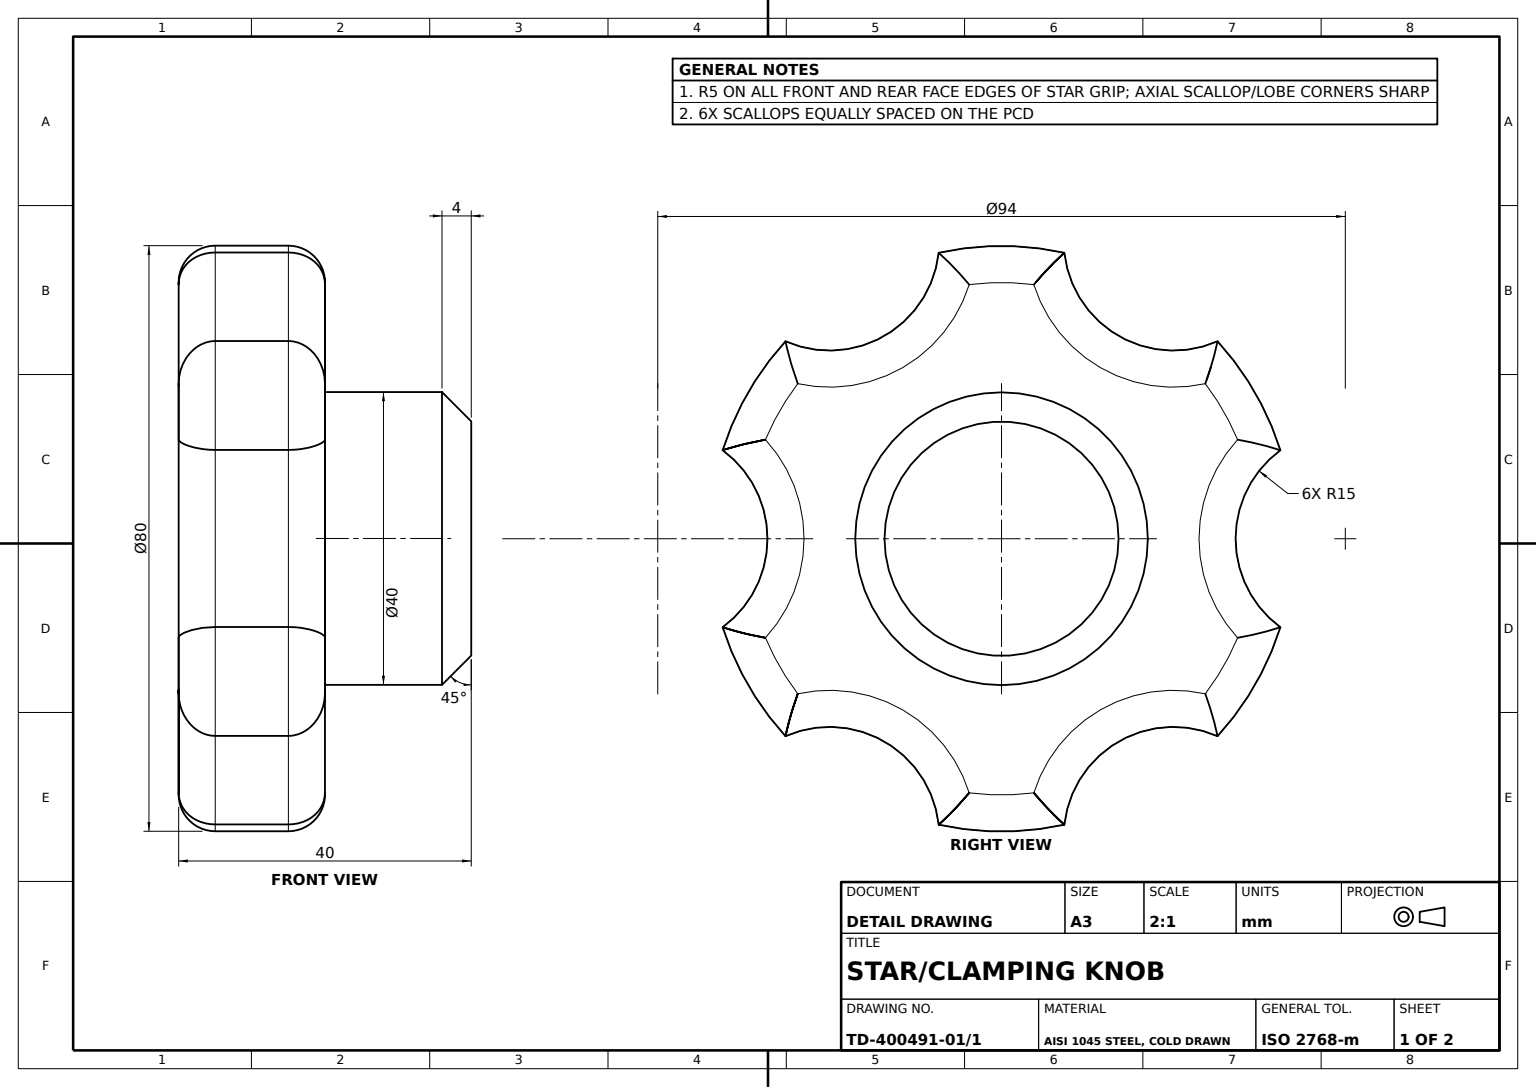
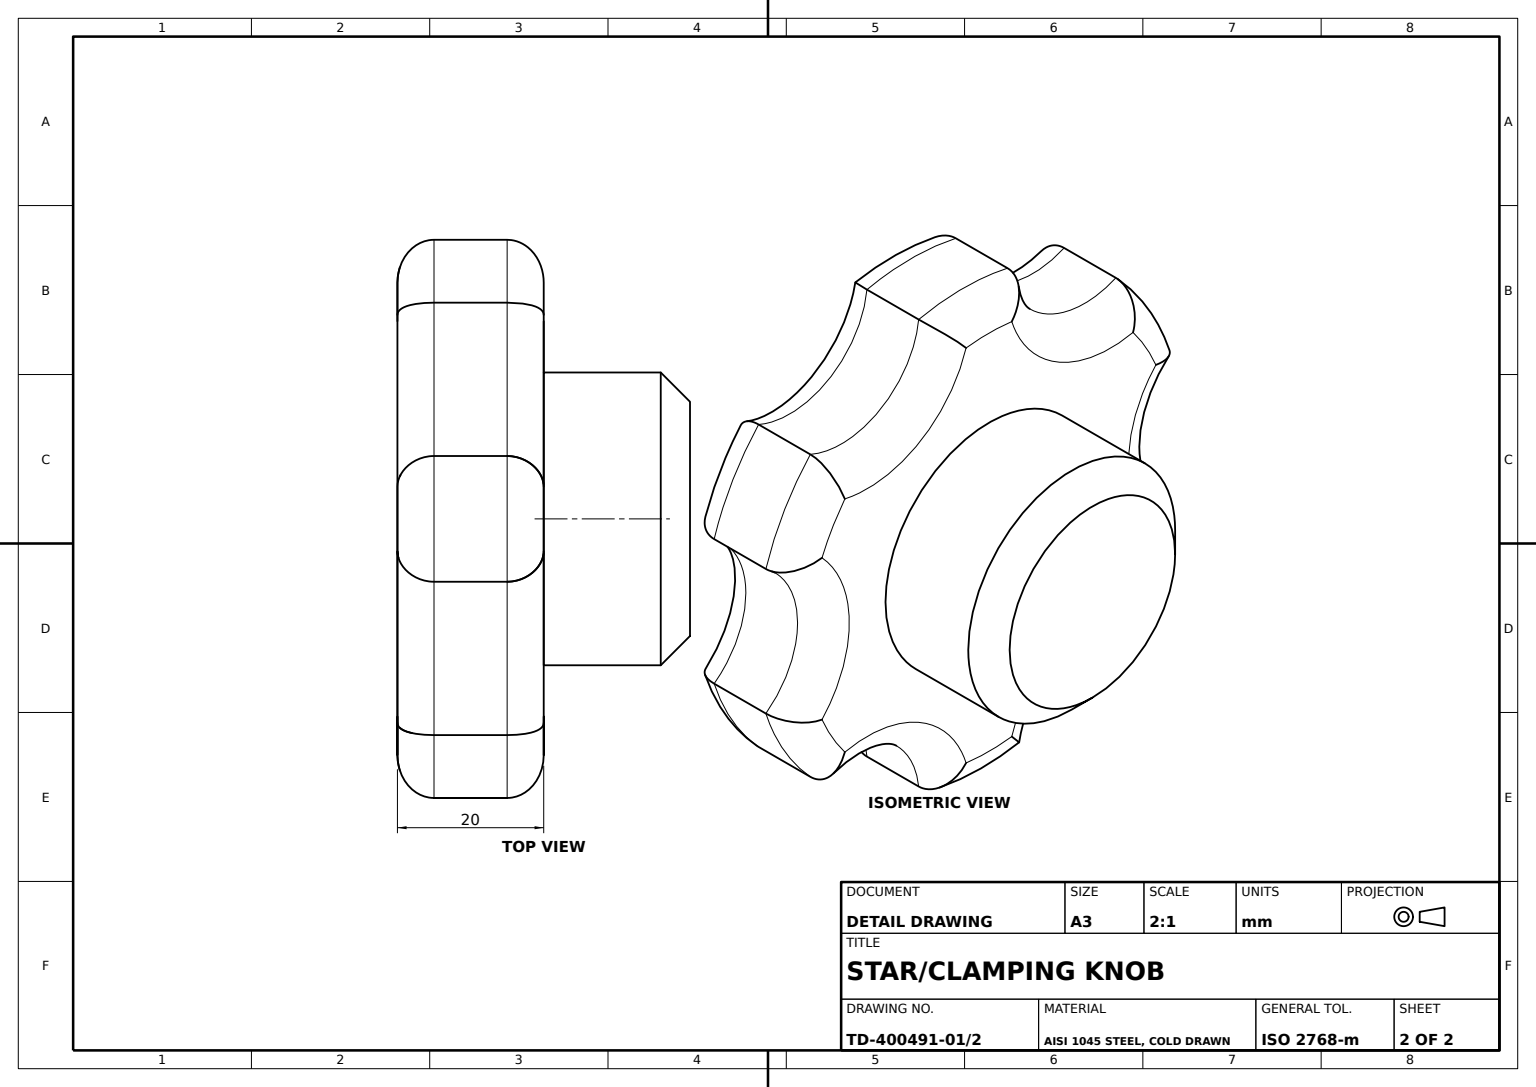
SolidWorks part; units mm, degrees
material "AISI 1045 Steel, cold drawn"
ref_plane "Front Plane" through (0, 0, 0) normal (0, 0, 1) x (1, 0, 0)
ref_plane "Top Plane" through (0, 0, 0) normal (0, 1, 0) x (1, 0, 0)
ref_plane "Right Plane" through (0, 0, 0) normal (1, 0, 0) x (0, 0, -1)
sketch "Star Profile Sketch" plane through (0, 0, 0) normal (0, 1, 0) x (1, 0, 0)
  line L0 (0, 62.3888) -> (0, -75.0628) construction
  line L1 (54.0303, -31.1944) -> (-65.0063, 37.5314) construction
  line L2 (-54.0303, -31.1944) -> (65.0063, 37.5314) construction
  circle A0 centre (0, 0) radius 47 construction
  arc A1 (-12.0947, 38.1277) -> (-26.9722, 29.5381) centre (0, 0) ccw
  arc A2 (-12.0947, 38.1277) -> (12.0947, 38.1277) centre (0, 47) ccw
  arc A3 (26.9722, 29.5381) -> (39.0669, 8.5895) centre (40.7032, 23.5) ccw
  arc A4 (39.0669, -8.5895) -> (26.9722, -29.5381) centre (40.7032, -23.5) ccw
  arc A5 (12.0947, -38.1277) -> (-12.0947, -38.1277) centre (0, -47) ccw
  arc A6 (-26.9722, -29.5381) -> (-39.0669, -8.5895) centre (-40.7032, -23.5) ccw
  arc A7 (-39.0669, 8.5895) -> (-26.9722, 29.5381) centre (-40.7032, 23.5) ccw
  arc A8 (-39.0669, 8.5895) -> (-39.0669, -8.5895) centre (0, 0) ccw
  arc A9 (-26.9722, -29.5381) -> (-12.0947, -38.1277) centre (0, 0) ccw
  arc A10 (12.0947, -38.1277) -> (26.9722, -29.5381) centre (0, 0) ccw
  arc A11 (39.0669, -8.5895) -> (39.0669, 8.5895) centre (0, 0) ccw
  arc A12 (26.9722, 29.5381) -> (12.0947, 38.1277) centre (0, 0) ccw
  point P12 (0, 0)
  point P18 (0.2527, 0)
  point P31 (0, 0)
  dimension "D1" = 94
  dimension "D3" = 80
  dimension "D4" = 15
  dimension "D6" = 0.2527
  dimension "D2" = 3
  dimension "D5" = 6
extrude "Star Grip Body" add sketch "Star Profile Sketch" along normal blind 20
fillet "Grip Edge Fillet R5" radius 5 24 edges at (0, 0, -32) (-20, 0, -34.641) (-27.7128, 0, -16) (-40, 0, 0) (-27.7128, 0, 16) (-20, 0, 34.641) (0, 0, 32) (20, 0, 34.641) (27.7128, 0, 16) (40, 0, 0) (27.7128, 0, -16) (20, 0, -34.641) (27.7128, 20, -16) (40, 20, 0) (27.7128, 20, 16) (20, 20, 34.641) (0, 20, 32) (-20, 20, 34.641) (-27.7128, 20, 16) (-40, 20, 0) (-27.7128, 20, -16) (-20, 20, -34.641) (0, 20, -32) (20, 20, -34.641)
sketch "Hub Sketch Ø40" plane through (0, 20, 0) normal (0, 1, 0) x (1, 0, 0)
  circle A0 centre (0, 0) radius 20
  dimension "D1" = 40
extrude "Hub Ø40" add sketch "Hub Sketch Ø40" along normal blind 20
chamfer "Hub Top Chamfer 4x45°" distance 4 angle 45 1 edges at (0, 40, 20)
